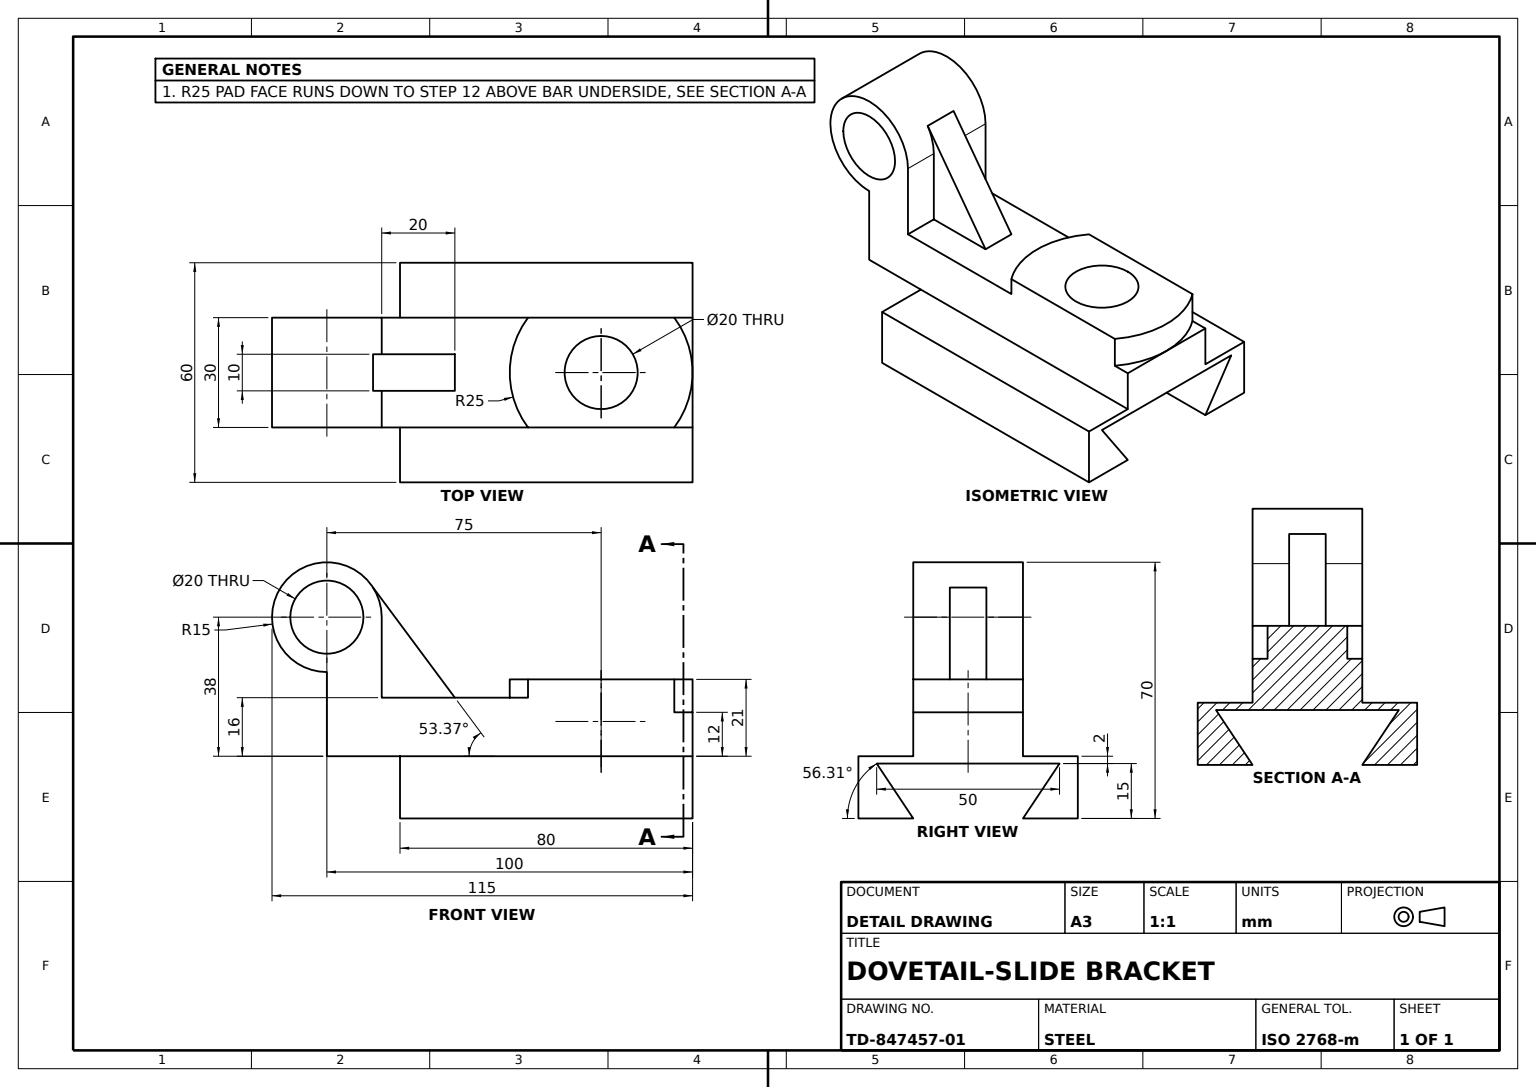
from build123d import *

# Parameters (mm, degrees)
SLOTTED_BASE_BLOCK_DEPTH = 80
PIVOT_PAD_SKETCH_R       = 25
PIVOT_PAD_50_DEPTH       = 21
UPPER_BAR_SKETCH_W       = 30
UPPER_BAR_SKETCH_H       = 12
UPPER_BAR_DEPTH          = 100
THROUGH_SLOT_PROFILE_W   = 15
THROUGH_SLOT_PROFILE_H   = 21
THROUGH_SLOT_CUT_DEPTH   = 100
EYE_LUG_PROFILE_R        = 10
RAISED_EYE_LUG_DEPTH     = 15
LUG_SUPPORT_RIB_REACH    = 132.131
LUG_RIB_SKETCH_WALL_W    = 299.76392147
LUG_RIB_SKETCH_WALL_H    = 10
PAD_HOLE_SKETCH_R        = 10
PAD_HOLE_20_DEPTH        = 30


with BuildPart() as part:
    # Base Block Profile → Slotted Base Block (new body)
    with BuildSketch(Plane(origin=(0, 0, 0), x_dir=(0, 0, -1), z_dir=(1, 0, 0))):
        Polygon((30, 0), (-30, 0), (-30, -17), (-15, -17), (-25, -2), (25, -2), (15, -17), (30, -17), align=None)
    extrude(amount=-SLOTTED_BASE_BLOCK_DEPTH)

    # Pivot Pad Sketch → Pivot Pad Ø50 (add)
    with BuildSketch(Plane(origin=(0, 0, 0), x_dir=(1, 0, 0), z_dir=(0, 1, 0))):
        with Locations((-25, 0)):
            Circle(PIVOT_PAD_SKETCH_R)
    extrude(amount=PIVOT_PAD_50_DEPTH)

    # Upper Bar Sketch → Upper Bar (add)
    with BuildSketch(Plane(origin=(0, 0, 0), x_dir=(0, 0, -1), z_dir=(1, 0, 0))):
        with Locations((0, 6)):
            Rectangle(UPPER_BAR_SKETCH_W, UPPER_BAR_SKETCH_H)
    extrude(amount=-UPPER_BAR_DEPTH)

    # Through Slot Profile → Through Slot Cut (cut)
    with BuildSketch(Plane(origin=(0, 0, 0), x_dir=(0, 0, -1), z_dir=(1, 0, 0))):
        with Locations((-22.5, 10.5)):
            Rectangle(THROUGH_SLOT_PROFILE_W, THROUGH_SLOT_PROFILE_H)
        with Locations((22.5, 10.5)):
            Rectangle(THROUGH_SLOT_PROFILE_W, THROUGH_SLOT_PROFILE_H)
    extrude(amount=-THROUGH_SLOT_CUT_DEPTH, mode=Mode.SUBTRACT)

    # Eye Lug Profile → Raised Eye Lug (add, symmetric)
    with BuildSketch(Plane.XY):
        with BuildLine():
            Line((-85, 16), (-85, 38))
            ThreePointArc((-85, 38), (-110.606601718, 48.606601718), (-100, 23))
            Line((-100, 23), (-100, 12))
            Line((-100, 12), (-45, 12))
            Line((-45, 12), (-45, 16))
            Line((-45, 16), (-85, 16))
        make_face()
        with Locations((-100, 38)):
            Circle(EYE_LUG_PROFILE_R, mode=Mode.SUBTRACT)
    extrude(amount=RAISED_EYE_LUG_DEPTH, both=True)

    # Lug Rib Sketch wall → Lug Support Rib (add, up to next)
    with BuildSketch(Plane(origin=(-76.186743425, 31.048801232, 0), x_dir=(0.596586314149, -0.802548920484, 0), z_dir=(0.802548920484, 0.596586314149, 0)), mode=Mode.PRIVATE) as lug_support_rib_sk1:
        Rectangle(LUG_RIB_SKETCH_WALL_W, LUG_RIB_SKETCH_WALL_H)
    lug_support_rib_tool1 = extrude(lug_support_rib_sk1.sketch, amount=-LUG_SUPPORT_RIB_REACH, mode=Mode.PRIVATE) - part.part
    add(lug_support_rib_tool1.solids().sort_by_distance((-76.186743425, 31.048801232, 0))[0])

    # Pad Hole Sketch → Pad Hole Ø20 (cut)
    with BuildSketch(Plane(origin=(0, 21, 0), x_dir=(1, 0, 0), z_dir=(0, 1, 0))):
        with Locations(Location((-25, 0, 0), (0, 0, 270))):
            Circle(PAD_HOLE_SKETCH_R)
    extrude(amount=-PAD_HOLE_20_DEPTH, mode=Mode.SUBTRACT)


solid = part.part
